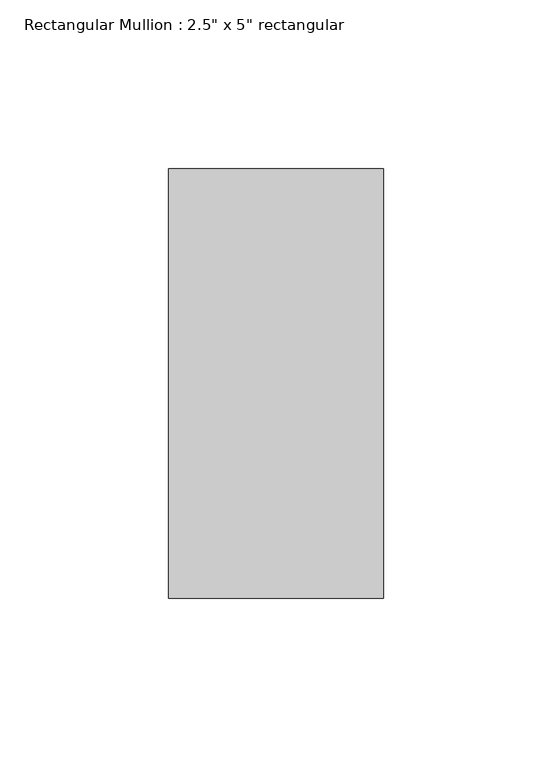
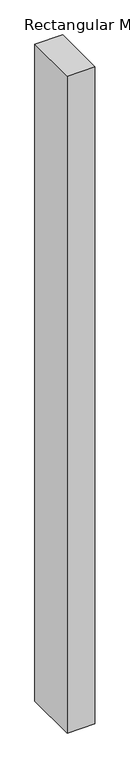
"""IFC4 building model written with IfcOpenShell, lengths in millimetres: member geometry."""

from ifc_helpers import new_model, si_unit, frame, origin, place, context, project, spatial, polyline, outline, extrude, source, transform, mapped, element, save


def member_623289aa(model_context):
    return source(origin(), model_context, "Body", "SweptSolid", [
        extrude(outline(polyline([(0.0, 63.5), (0.0, -63.5), (-63.5, -63.5), (-63.5, 63.5), (0.0, 63.5)])), frame((0.0, 0.0, -1586.2856263), z_axis=(0.0, 0.0, 1.0), x_axis=(1.0, 0.0, 0.0)), (0.0, 0.0, 1.0), 1586.2856263),
    ])


if __name__ == "__main__":
    model = new_model("IFC4")
    model_context = context("Model", 3, world=origin())
    ifc_project = project(units=[si_unit("LENGTHUNIT", "METRE", prefix="MILLI")], contexts=[model_context])
    site = spatial("IfcSite", under=ifc_project)
    building = spatial("IfcBuilding", under=site)
    placement = place(None, origin())
    member_shape = member_623289aa(model_context)
    element("IfcMember", 1, ObjectType="Rectangular Mullion : 2.5\" x 5\" rectangular", at=placement, inside=building, context=model_context, shape_type="MappedRepresentation", body=[
        mapped(member_shape, transform((0.0, 0.0, 0.0), x_axis=(1.0, 0.0, 0.0), y_axis=(0.0, 1.0, 0.0), z_axis=(0.0, 0.0, 1.0))),
    ])
    save(model, "model.ifc")

# Revit data of these elements
# Type "Rectangular Mullion : 2.5\" x 5\" rectangular"
#   built-in parameter 1007304 = 0.416667 (stored number, unit not read)
#   built-in parameter 1007301 = 0.104167 (stored number, unit not read)
#   built-in parameter 1007300 = 0.104167 (stored number, unit not read)
# Element 1 (IfcMember, "Rectangular Mullion : 2.5\" x 5\" rectangular")
#   Materials on its faces: "Aluminum"
# Materials
#   "Aluminum": class "Metal", colour RGB 247 247 247, transparency 0, Description = "Aluminum 6061", Cost = 0
